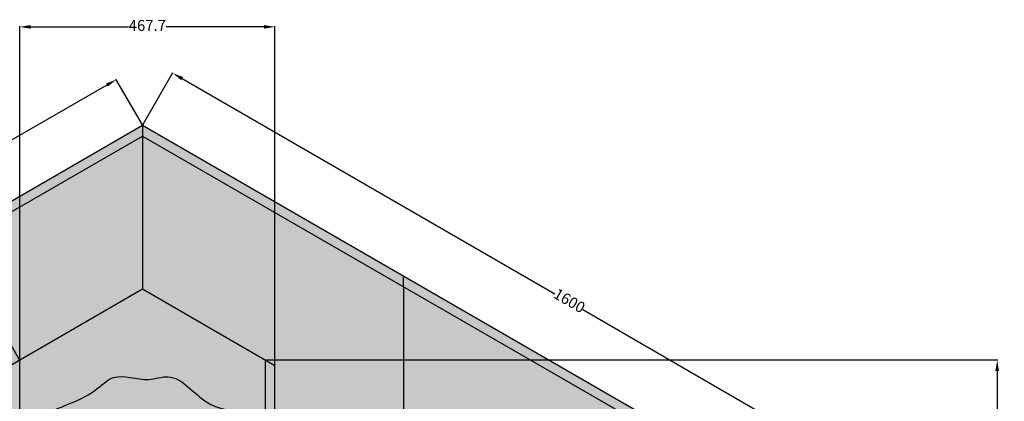
# Model space of a CAD drawing. Units: millimetres. Extents: x 78378 to 86415, y 148682 to 152721.
# Tile 16 of 18: x 80164 to 81968, y 151749 to 152448. Entities that reach past the tile are written whole.
import ezdxf

# ---------------------------------------------------------------- set-up
doc = ezdxf.new("R2010")
doc.units = ezdxf.units.MM
for name, color, linetype, lineweight in [('A-ANNO-DIMS', 2, 'Continuous', 18), ('A-FURN', 4, 'Continuous', 25), ('A-FURN-PATT', 32, 'Continuous', 13)]:
    doc.layers.add(name, color=color, linetype=linetype, lineweight=lineweight)
doc.styles.get("Standard").update_dxf_attribs({"font": 'arial.ttf'})
doc.dimstyles.new('ISO-25', dxfattribs={"dimtxt": 20, "dimasz": 20, "dimexe": 1.25, "dimexo": 0.625, "dimtad": 0, "dimdec": 1, "dimtxsty": 'Standard', "dimcen": 2.5, "dimadec": 0, "dimazin": 0, "dimtfac": 1, "dimtdec": 1, "dimtmove": 0, "dimatfit": 3, "dimfxl": 1, "dimarcsym": 0})

# ---------------------------------------------------------------- blocks, each defined once
blk = doc.blocks.new('*D2')
at = {"layer": 'A-ANNO-DIMS', "color": 0, "lineweight": -2, "transparency": 16777216}
for p, q in [((80324, 152328.4), (79430.3, 151812.5)), ((80389.2, 152255.5), (80340.7, 152339.5)), ((78540, 151298.4), (79377.3, 151781.8)), ((78570.5, 151205.5), (78522.1, 151289.5))]:
    blk.add_line(p, q, dxfattribs=at)
at = {"layer": 'A-ANNO-DIMS', "color": 0, "transparency": 16777216}
for points in [[(80322.4, 152331.3), (80325.7, 152325.6), (80341.3, 152338.4)], [(78538.3, 151301.3), (78541.7, 151295.6), (78522.7, 151288.4)]]:
    blk.add_solid(points, dxfattribs=at)
at = {"layer": 'Defpoints', "color": 0, "transparency": 16777216}
for p in [(80341.3, 152338.4), (80389.5, 152255), (78570.9, 151205)]:
    blk.add_point(p, dxfattribs=at)
at = {"layer": 'A-ANNO-DIMS', "color": 0, "transparency": 16777216, "insert": (79403.8, 151797.2), "char_height": 20, "attachment_point": 5, "rotation": 30}
blk.add_mtext('2100', dxfattribs=at)
blk = doc.blocks.new('*D3')
at = {"layer": 'A-ANNO-DIMS', "color": 0, "lineweight": -2, "transparency": 16777216}
for p, q in [((80389.8, 152255.5), (80445.2, 152351.4)), ((80461.9, 152340.3), (81144.7, 151946.1)), ((81812.9, 151560.3), (81195.8, 151916.6)), ((81775.5, 151455.5), (81830.8, 151551.4))]:
    blk.add_line(p, q, dxfattribs=at)
at = {"layer": 'A-ANNO-DIMS', "color": 0, "transparency": 16777216}
for points in [[(80463.5, 152343.2), (80460.2, 152337.4), (80444.5, 152350.3)], [(81814.5, 151563.2), (81811.2, 151557.4), (81830.2, 151550.3)]]:
    blk.add_solid(points, dxfattribs=at)
at = {"layer": 'Defpoints', "color": 0, "transparency": 16777216}
for p in [(80389.5, 152255), (81830.2, 151550.3), (81775.2, 151455)]:
    blk.add_point(p, dxfattribs=at)
at = {"layer": 'A-ANNO-DIMS', "color": 0, "transparency": 16777216, "insert": (81170.2, 151931.4), "char_height": 20, "attachment_point": 5, "rotation": 330}
blk.add_mtext('1600', dxfattribs=at)
blk = doc.blocks.new('*D17')
at = {"layer": 'A-ANNO-DIMS', "color": 0, "lineweight": -2, "transparency": 16777216}
for p, q in [((80164, 151825.5), (80073.7, 151982)), ((80057, 151970.9), (79823.5, 151836.1)), ((79550.4, 151678.4), (79783.9, 151813.2)), ((79622.8, 151513), (79532.5, 151669.5))]:
    blk.add_line(p, q, dxfattribs=at)
at = {"layer": 'A-ANNO-DIMS', "color": 0, "transparency": 16777216}
for points in [[(80055.4, 151973.8), (80058.7, 151968), (80074.3, 151980.9)], [(79548.7, 151681.3), (79552.1, 151675.5), (79533.1, 151668.4)]]:
    blk.add_solid(points, dxfattribs=at)
at = {"layer": 'Defpoints', "color": 0, "transparency": 16777216}
for p in [(80074.3, 151980.9), (80164.3, 151825), (79623.1, 151512.5)]:
    blk.add_point(p, dxfattribs=at)
at = {"layer": 'A-ANNO-DIMS', "color": 0, "transparency": 16777216, "insert": (79803.7, 151824.6), "char_height": 20, "attachment_point": 5, "rotation": 30}
blk.add_mtext('625', dxfattribs=at)
blk = doc.blocks.new('*D30')
at = {"layer": 'A-ANNO-DIMS', "color": 0, "lineweight": -2, "transparency": 16777216}
for p, q in [((80615.3, 151825), (81956.4, 151825)), ((81955.2, 151805), (81955.2, 151487.6)), ((81955.2, 151125), (81955.2, 151442.4)), ((80615.3, 151105), (81956.4, 151105))]:
    blk.add_line(p, q, dxfattribs=at)
at = {"layer": 'A-ANNO-DIMS', "color": 0, "transparency": 16777216}
for points in [[(81951.8, 151805), (81958.5, 151805), (81955.2, 151825)], [(81951.8, 151125), (81958.5, 151125), (81955.2, 151105)]]:
    blk.add_solid(points, dxfattribs=at)
at = {"layer": 'Defpoints', "color": 0, "transparency": 16777216}
for p in [(80614.7, 151825), (81955.2, 151825), (80614.7, 151105)]:
    blk.add_point(p, dxfattribs=at)
at = {"layer": 'A-ANNO-DIMS', "color": 0, "transparency": 16777216, "insert": (81955.2, 151465), "char_height": 20, "attachment_point": 5, "rotation": 90}
blk.add_mtext('720', dxfattribs=at)
blk = doc.blocks.new('*D33')
at = {"layer": 'A-ANNO-DIMS', "color": 0, "lineweight": -2, "transparency": 16777216}
for p, q in [((80164.3, 151105.6), (80164.3, 152436.3)), ((80184.3, 152435), (80363.4, 152435)), ((80612, 152435), (80432.9, 152435)), ((80632, 151105.6), (80632, 152436.3))]:
    blk.add_line(p, q, dxfattribs=at)
at = {"layer": 'A-ANNO-DIMS', "color": 0, "transparency": 16777216}
for points in [[(80184.3, 152438.3), (80184.3, 152431.7), (80164.3, 152435)], [(80612, 152438.3), (80612, 152431.7), (80632, 152435)]]:
    blk.add_solid(points, dxfattribs=at)
at = {"layer": 'Defpoints', "color": 0, "transparency": 16777216}
for p in [(80632, 152435), (80164.3, 151105), (80632, 151105)]:
    blk.add_point(p, dxfattribs=at)
at = {"layer": 'A-ANNO-DIMS', "color": 0, "transparency": 16777216, "insert": (80398.2, 152435), "char_height": 20, "attachment_point": 5}
blk.add_mtext('467.7', dxfattribs=at)

msp = doc.modelspace()

# ---------------------------------------------------------------- hatches: boundary and pattern name
at = {"layer": 'A-FURN-PATT'}
h = msp.add_hatch(color=256, dxfattribs=at)
h.dxf.hatch_style = 1
h.paths.add_polyline_path([(80389.5131, 152235.0076), (80389.5131, 152255.0076), (79662.0518, 151835.0076), (79662.0518, 151815.0076)])
h.paths.add_polyline_path([(79662.0518, 151815.0076), (79662.0518, 151835.0076), (79099.1352, 151510.0076), (79099.1352, 151490.0076)])
h.paths.add_polyline_path([(79099.1352, 151490.0076), (79099.1352, 151510.0076), (78579.52, 151210.0076), (78596.8405, 151200.0076)])
h.paths.add_polyline_path([(80632.0002, 152115.0076), (80632.0002, 152095.0076), (80867.7794, 151958.8805), (80867.7794, 151978.8805)])
h.paths.add_polyline_path([(80389.5131, 152255.0076), (80389.5131, 152235.0076), (80632.0002, 152095.0076), (80632.0002, 152115.0076)])
h = msp.add_hatch(color=256, dxfattribs=at)
h.dxf.hatch_style = 1
h.paths.add_polyline_path([(78839.3276, 151040.0076), (78579.52, 151190.0076), (78579.52, 150470.0076), (78839.3276, 150320.0076)])
h.paths.add_polyline_path([(79073.1545, 150899.6469, 0.277779695), (79002.2645, 150996.3205, 0.791083931), (78917.9567, 150978.8719, 0.180448316), (78856.6481, 150853.0138), (78856.6481, 150350.6973), (79073.1545, 150484.318)])
h.paths.add_polyline_path([(79073.1545, 151175.0076), (78856.6481, 151050.0076), (78856.6481, 150853.0138, -0.180448316), (78917.9567, 150978.8719, -0.791083931), (79002.2645, 150996.3205, -0.277779695), (79073.1545, 150899.6469)])
h.paths.add_polyline_path([(79341.6224, 151350.0076), (79099.1352, 151490.0076), (78596.8405, 151200.0076), (78839.3276, 151060.0076)])
h.paths.add_polyline_path([(79904.5389, 151675.0076), (79662.0518, 151815.0076), (79099.1352, 151490.0076), (79341.6224, 151350.0076)])
h.paths.add_polyline_path([(80389.5131, 151955.0076), (80389.5131, 152235.0076), (79662.0518, 151815.0076), (79904.5389, 151675.0076)])
h.paths.add_polyline_path([(80389.5131, 151955.0076), (80164.3465, 151825.0076), (80164.3465, 151105.0076), (80614.6797, 151105.0076), (80614.6797, 151825.0076)])
edge = h.paths.add_edge_path(flags=16)
edge.add_spline(control_points=[(80216.308, 151728.251), (80227.1854, 151732.981), (80256.3301, 151745.6544), (80298.41, 151761.9595), (80340.2597, 151805.855), (80391.0771, 151782.0404), (80454.0396, 151805.7581), (80496.5007, 151742.4095), (80543.8218, 151733.4043), (80562.7182, 151729.8083)], knot_values=[0, 0, 0, 0, 35.543746761, 95.235753469, 136.367675126, 200.932981967, 236.726410811, 322.889934976, 380.170273667, 380.170273667, 380.170273667, 380.170273667], degree=3, periodic=0)
edge.add_line((80562.7182, 151729.8083), (80562.7182, 151165.0076))
edge.add_line((80562.7182, 151165.0076), (80216.308, 151165.0076))
edge.add_line((80216.308, 151165.0076), (80216.308, 151728.251))
h.paths.add_polyline_path([(80632.0002, 152095.0076), (80389.5131, 152235.0076), (80389.5131, 151955.0076), (80614.6797, 151825.0076), (80632.0002, 151815.0076)])
h.paths.add_polyline_path([(80867.7794, 151958.8805), (80632.0002, 152095.0076), (80632.0002, 151815.0076), (80632.0002, 151510.0076), (80867.7794, 151373.8805)])
h.paths.add_polyline_path([(80147.026, 151495.8203, 0.18918979), (80063.5671, 151597.7244, 0.788261355), (79979.2691, 151580.5832, 0.160726132), (79904.5389, 151413.5769), (79904.5389, 150955.0076), (80147.026, 151095.0076)])
h.paths.add_polyline_path([(80147.026, 151815.0076), (79904.5389, 151675.0076), (79904.5389, 151413.5769, -0.160726132), (79979.2691, 151580.5832, -0.788261355), (80063.5671, 151597.7244, -0.18918979), (80147.026, 151495.8203)])
h.paths.add_polyline_path([(79887.2184, 151645.0076), (79640.4011, 151502.5076), (79640.4011, 151262.3325, -0.160726132), (79715.1313, 151429.3387, -0.788261355), (79799.4294, 151446.48, -0.21290578), (79887.2184, 151328.7247)])
h.paths.add_polyline_path([(79799.4294, 151446.48, 0.788261355), (79715.1313, 151429.3387, 0.160726132), (79640.4011, 151262.3325), (79640.4011, 150822.5076), (79887.2184, 150965.0076), (79887.2184, 151328.7247, 0.21290578)])
h.paths.add_polyline_path([(79605.7601, 151482.5076), (79358.9429, 151340.0076), (79358.9429, 151100.0701, -0.160726132), (79433.6731, 151267.0764, -0.788261355), (79517.9711, 151284.2176, -0.21290578), (79605.7601, 151166.4623)])
h.paths.add_polyline_path([(79605.7601, 151166.4623, 0.21290578), (79517.9711, 151284.2176, 0.788261355), (79433.6731, 151267.0764, 0.160726132), (79358.9429, 151100.0701), (79358.9429, 150742.9831), (79419.0877, 150694.7323), (79605.7601, 150802.5076)])
edge = h.paths.add_edge_path(flags=0)
edge.add_spline(control_points=[(81152.4356, 151098.7676), (81105.7208, 151145.9466), (81038.6136, 151213.7208), (80882.3866, 151214.1938), (80797.4434, 151311.2997), (80711.8686, 151340.3754), (80681.7691, 151350.6023)], knot_values=[0, 0, 0, 0, 188.233441, 270.4032752, 445.451792012, 540.428588287, 540.428588287, 540.428588287, 540.428588287], degree=3, periodic=0)
edge.add_line((80683.4538, 151350.0269), (80683.4538, 151104.8792))
edge.add_line((80683.4538, 151104.8792), (81152.4356, 150851.399))
edge.add_line((81152.4356, 150851.399), (81152.4356, 151098.7676))
edge = h.paths.add_edge_path(flags=0)
edge.add_spline(control_points=[(80912.9018, 151027.1103), (80892.3742, 151034.1027), (80860.1663, 151045.0739), (80835.5097, 151068.1214), (80826.5679, 151076.4797)], knot_values=[0, 0, 0, 0, 63.98405104, 100.391424282, 100.391424282, 100.391424282, 100.391424282], degree=3, periodic=0)
edge.add_arc((80830.0414, 151081.2992), 5.9407, 100.9277276, 234.2187381, ccw=False)
edge.add_spline(control_points=[(80828.9152, 151087.1322), (80837.857, 151078.7739), (80862.5136, 151055.7263), (80894.7215, 151044.7552), (80915.2491, 151037.7628)], knot_values=[0, 0, 0, 0, 36.407373242, 100.391424282, 100.391424282, 100.391424282, 100.391424282], degree=3, periodic=0)
edge.add_arc((80914.7882, 151032.2795), 5.5026, -107.9540399, 85.195579, ccw=False)
h.paths.add_polyline_path([(81238.218, 151110.0076), (80632.0002, 151460.0076), (80632.0002, 151105.0076), (81238.218, 150755.0076)])
edge = h.paths.add_edge_path(flags=16)
edge.add_line((81152.4356, 150851.399), (80683.4538, 151104.8792))
edge.add_line((80683.4538, 151104.8792), (80683.4538, 151350.0279))
edge.add_spline(control_points=[(80681.7691, 151350.6023), (80711.8686, 151340.3754), (80797.4434, 151311.2997), (80882.3866, 151214.1938), (81038.6136, 151213.7208), (81105.7208, 151145.9466), (81152.4356, 151098.7676)], knot_values=[0, 0, 0, 0, 94.976796275, 270.025313088, 352.195147288, 540.428588287, 540.428588287, 540.428588287, 540.428588287], degree=3, periodic=0)
edge.add_line((81152.4356, 151098.7676), (81152.4356, 150851.399))
edge = h.paths.add_edge_path(flags=0)
edge.add_spline(control_points=[(80912.9018, 151027.1103), (80892.3742, 151034.1027), (80860.1663, 151045.0739), (80835.5097, 151068.1214), (80826.5679, 151076.4797)], knot_values=[0, 0, 0, 0, 63.98405104, 100.391424282, 100.391424282, 100.391424282, 100.391424282], degree=3, periodic=0)
edge.add_arc((80830.0414, 151081.2992), 5.9407, 100.9277276, 234.2187381, ccw=False)
edge.add_spline(control_points=[(80828.9152, 151087.1322), (80837.857, 151078.7739), (80862.5136, 151055.7263), (80894.7215, 151044.7552), (80915.2491, 151037.7628)], knot_values=[0, 0, 0, 0, 36.407373242, 100.391424282, 100.391424282, 100.391424282, 100.391424282], degree=3, periodic=0)
edge.add_arc((80914.7882, 151032.2795), 5.5026, -107.7417882, 85.195579, ccw=False)
h.paths.add_polyline_path([(81498.0256, 151255.0076), (81238.218, 151110.0076), (81238.218, 150755.0076), (81498.0256, 150905.0076)])
edge = h.paths.add_edge_path(flags=16)
edge.add_spline(control_points=[(81152.4356, 151098.7676), (81105.7208, 151145.9466), (81038.6136, 151213.7208), (80882.3866, 151214.1938), (80797.4434, 151311.2997), (80711.8686, 151340.3754), (80681.7691, 151350.6023)], knot_values=[0, 0, 0, 0, 188.233441, 270.4032752, 445.451792012, 540.428588287, 540.428588287, 540.428588287, 540.428588287], degree=3, periodic=0)
edge.add_line((80683.4538, 151350.0279), (80683.4538, 151104.8792))
edge.add_line((80683.4538, 151104.8792), (81152.4356, 150851.399))
edge.add_line((81152.4356, 150851.399), (81152.4356, 151098.7676))
h.paths.add_polyline_path([(81453.9904, 151280.4314), (80867.7794, 151618.8805), (80867.7794, 151373.8805), (81238.218, 151160.0076)])
edge = h.paths.add_edge_path(flags=16)
edge.add_line((81189.2304, 151297.6373), (81114.4166, 151300.2154))
edge.add_arc((81412.0967, 151394.0167), 312.1092, 179.7569303, 197.4900342, ccw=False)
edge.add_ellipse((81154.0183, 151392.0436), major_axis=(-54.0264, 3.6301), ratio=0.221796934, start_angle=0, end_angle=0.3517985, ccw=False)
edge.add_ellipse((81154.0183, 151392.0436), major_axis=(-54.0264, 3.6301), ratio=0.221796934, start_angle=180, end_angle=360, ccw=False)
edge.add_spline(control_points=[(81196.1844, 151321.9476), (81224.9802, 151347.1455), (81266.8846, 151383.8144), (81222.0354, 151387.0304), (81208.0056, 151388.0364)], knot_values=[0, 0, 0, 0, 75.091751734, 109.275804387, 109.275804387, 109.275804387, 109.275804387], degree=3, periodic=0)
edge.add_arc((80751.9112, 151435.6145), 458.5693, 342.4891602, 345.646172, ccw=False)
edge = h.paths.add_edge_path(flags=0)
edge.add_spline(control_points=[(81196.6193, 151323.657), (81197.893, 151324.7717), (81199.1654, 151325.8858), (81209.0233, 151334.5343), (81217.3959, 151341.9835), (81228.0928, 151352.5012), (81231.3883, 151355.9524), (81236.9493, 151362.4395), (81239.214, 151365.4773), (81241.4987, 151369.416), (81242.064, 151370.5542), (81242.9187, 151372.6971), (81243.2076, 151373.7015), (81243.5012, 151375.5539), (81243.5065, 151376.4), (81243.2432, 151377.9407), (81242.9775, 151378.6373), (81242.1402, 151379.937), (81241.5659, 151380.5416), (81240.2039, 151381.533), (81239.4963, 151381.9384), (81237.0619, 151383.0663), (81235.0242, 151383.6999), (81230.352, 151384.7569), (81227.7173, 151385.1826), (81221.9118, 151385.9145), (81218.7193, 151386.2133), (81213.7912, 151386.6115), (81212.1252, 151386.7359), (81209.6196, 151386.9181), (81208.7865, 151386.9779), (81207.9009, 151387.0432)], knot_values=[0.015487437, 0.015487437, 0.015487437, 0.015487437, 3.337879569, 3.337879569, 25.851306242, 25.851306242, 37.52811308, 37.52811308, 49.204919918, 49.204919918, 54.285093801, 54.285093801, 59.365267683, 59.365267683, 64.445441566, 64.445441566, 69.525615449, 69.525615449, 74.605789331, 74.605789331, 78.493667847, 78.493667847, 86.255670953, 86.255670953, 94.017674059, 94.017674059, 102.202265559, 102.202265559, 106.294561309, 106.294561309, 108.325221747, 108.325221747, 108.325221747, 108.325221747], degree=3, periodic=0)
edge = h.paths.add_edge_path(flags=16)
edge.add_arc((81034.1732, 151350.4693), 42.5822, 231.2679035, 306.151846, ccw=False)
edge.add_line((81007.5303, 151317.2517), (81007.5303, 151395.181))
edge.add_ellipse((81033.412, 151394.7791), major_axis=(-25.8816, 0.4538), ratio=0.23894509, start_angle=0, end_angle=0.1147075, ccw=False)
edge.add_ellipse((81033.412, 151394.7791), major_axis=(-25.8816, 0.4538), ratio=0.23894509, start_angle=181.1677709, end_angle=358.9476457, ccw=False)
edge.add_ellipse((81033.412, 151395.7791), major_axis=(-25.8816, 0.4538), ratio=0.23894509, start_angle=180, end_angle=360.1147075, ccw=False)
edge.add_ellipse((81033.412, 151395.7791), major_axis=(-25.8816, 0.4538), ratio=0.23894509, start_angle=178.9476457, end_angle=180, ccw=False)
edge.add_line((81059.2936, 151395.1778), (81059.2936, 151394.3772))
edge.add_ellipse((81033.412, 151394.7791), major_axis=(-25.8816, 0.4538), ratio=0.23894509, start_angle=180, end_angle=180.1147075, ccw=False)
edge.add_ellipse((81033.412, 151394.7791), major_axis=(-25.8816, 0.4538), ratio=0.23894509, start_angle=3.6903098, end_angle=176.4406503, ccw=False)
edge.add_line((81059.2936, 151393.3388), (81059.2936, 151316.086))
h.paths.add_polyline_path([(80951.9355, 151343.9568), (80909.6838, 151362.4635), (80904.0219, 151443.9615, -0.381333076), (80987.2169, 151411.3717)], flags=16)
h = msp.add_hatch(color=256, dxfattribs=at)
h.dxf.hatch_style = 1
h.paths.add_polyline_path([(80867.7794, 151978.8805), (80867.7794, 151958.8805), (81766.4935, 151440.0076), (81766.4935, 150140.0076), (81775.1537, 150135.0076), (81775.1537, 151455.0076)])
h = msp.add_hatch(color=256, dxfattribs=at)
h.dxf.hatch_style = 1
h.paths.add_polyline_path([(80389.8136, 150935.1811), (80389.5131, 151105.0076), (80164.3465, 151105.0076), (79904.5389, 150955.0076), (79433.5848, 150683.1022), (79459.4128, 150662.3818), (79243.9048, 150537.9582), (79160.4069, 150518.1674), (78839.3276, 150320.0076), (78579.52, 150470.0076), (78570.8597, 150475.0076), (78570.8597, 150465.0076), (78570.8597, 149885.0076)])
h.paths.add_polyline_path([(80086.4042, 150460.0076), (79826.5966, 150610.0076), (78570.8597, 149885.0076), (78830.6674, 149735.0076)])
h.paths.add_polyline_path([(79540.8001, 150161.0557), (79217.3967, 149974.3386), (78980.9166, 150110.8705), (79304.32, 150297.5875)], flags=16)
h.paths.add_polyline_path([(79506.159, 150161.0557), (79217.3967, 149994.3386), (79015.5576, 150110.8705), (79304.32, 150277.5875)], flags=0)
edge = h.paths.add_edge_path(flags=0)
edge.add_arc((79247.8636, 150177.1541), 137.9799, 256.0025928, 293.5594109)
edge.add_arc((79240.7671, 150078.2605), 68.0855, 336.099104, 387.3696877)
edge.add_ellipse((79258.3074, 150109.4852), major_axis=(-42.6234, -1.6591), ratio=0.160428429, start_angle=0, end_angle=179.0977279, ccw=False)
edge.add_arc((79285.2112, 150074.2509), 77.2096, 155.1233104, 203.6557939)
edge = h.paths.add_edge_path(flags=0)
edge.add_ellipse((79258.6958, 150110.8297), major_axis=(-42.6234, -1.6591), ratio=0.160428429, start_angle=350.6039412, end_angle=356.2289762)
edge.add_line((79219.169, 150111.8937), (79218.3268, 150109.4141))
edge.add_arc((79262.4675, 150032.9602), 88.2813, 112.3931229, 120, ccw=False)
h.paths.add_polyline_path([(79287.0625, 150086.9703, -0.247702064), (79288.1967, 150077.2955, -0.390476513), (79265.4731, 150072.5438, -0.487261526), (79264.079, 150082.3769, 0.395604326)], flags=0)
h.paths.add_polyline_path([(80389.5131, 150935.0076), (79826.5966, 150610.0076), (80086.4042, 150460.0076), (80692.622, 150460.0076), (80952.4296, 150610.0076)])
edge = h.paths.add_edge_path(flags=16)
edge.add_ellipse((80392.4466, 150825.601), major_axis=(-133.0757, 7.722), ratio=0.42449957, start_angle=0, end_angle=360)
edge = h.paths.add_edge_path(flags=0)
edge.add_spline(control_points=[(80269.3541, 150832.7436), (80269.2919, 150831.672), (80269.3503, 150830.5922), (80269.7341, 150828.3361), (80270.0612, 150827.1587), (80271.0461, 150824.6748), (80271.7052, 150823.3692), (80273.4061, 150820.6503), (80274.4481, 150819.2381), (80276.9366, 150816.3509), (80278.3828, 150814.8762), (80282.5858, 150811.0913), (80285.6261, 150808.7701), (80292.6031, 150804.2267), (80296.5388, 150802.0041), (80305.195, 150797.7581), (80309.9151, 150795.7344), (80320.0112, 150791.96), (80325.387, 150790.2092), (80339.2162, 150786.315), (80347.9578, 150784.3563), (80366.0679, 150781.2568), (80375.4359, 150780.1158), (80394.3093, 150778.7158), (80403.8142, 150778.4568), (80422.4656, 150778.8319), (80431.6115, 150779.4662), (80449.0608, 150781.5838), (80457.3636, 150783.0675), (80472.6699, 150786.7766), (80479.6726, 150789.0033), (80490.1894, 150793.2813), (80494.1268, 150795.1967), (80501.0146, 150799.1885), (80503.9632, 150801.2651), (80508.2066, 150804.9015), (80509.73, 150806.4609), (80512.1996, 150809.4942), (80513.1456, 150810.9657), (80514.4291, 150813.5431), (80514.8436, 150814.6688), (80515.3984, 150816.8625), (80515.5405, 150817.9315), (80515.5801, 150820.098), (80515.4773, 150821.1978), (80514.9905, 150823.5062), (80514.6047, 150824.7154), (80513.4854, 150827.2641), (80512.7511, 150828.6027), (80510.8872, 150831.3809), (80509.7578, 150832.8196), (80507.0873, 150835.7513), (80505.5466, 150837.2439), (80501.0624, 150841.0944), (80497.8199, 150843.4576), (80490.4174, 150848.062), (80486.2582, 150850.3037), (80477.1448, 150854.5643), (80472.1909, 150856.5835), (80461.6275, 150860.3245), (80456.0182, 150862.0465), (80441.7332, 150865.8127), (80432.7885, 150867.6675), (80414.3391, 150870.5317), (80404.8349, 150871.5411), (80385.7707, 150872.6572), (80376.2113, 150872.764), (80357.5444, 150872.0728), (80348.4375, 150871.2748), (80331.1682, 150868.83), (80323.0064, 150867.1827), (80309.472, 150863.5363), (80303.8628, 150861.6593), (80293.8018, 150857.5401), (80289.3512, 150855.2969), (80282.7757, 150851.2345), (80280.3473, 150849.4579), (80276.2606, 150845.9127), (80274.604, 150844.1458), (80272.3157, 150841.1243), (80271.5358, 150839.8454), (80270.3496, 150837.3879), (80269.9417, 150836.2101), (80269.5065, 150834.2815), (80269.3988, 150833.5143), (80269.3541, 150832.7436)], knot_values=[0, 0, 0, 0, 0.09750046, 0.09750046, 0.19500092, 0.19500092, 0.292501379, 0.292501379, 0.390001839, 0.390001839, 0.487502299, 0.487502299, 0.638803224, 0.638803224, 0.790104149, 0.790104149, 0.941405074, 0.941405074, 1.092705999, 1.092705999, 1.312817101, 1.312817101, 1.532928203, 1.532928203, 1.753039304, 1.753039304, 1.973150406, 1.973150406, 2.193261508, 2.193261508, 2.413372609, 2.413372609, 2.569860633, 2.569860633, 2.726348657, 2.726348657, 2.844186582, 2.844186582, 2.962024507, 2.962024507, 3.060233876, 3.060233876, 3.158443245, 3.158443245, 3.256652615, 3.256652615, 3.354861984, 3.354861984, 3.453071354, 3.453071354, 3.551280723, 3.551280723, 3.649490093, 3.649490093, 3.80392773, 3.80392773, 3.958365368, 3.958365368, 4.112803006, 4.112803006, 4.267240644, 4.267240644, 4.489203495, 4.489203495, 4.711166346, 4.711166346, 4.933129197, 4.933129197, 5.155092048, 5.155092048, 5.3770549, 5.3770549, 5.557853609, 5.557853609, 5.738652318, 5.738652318, 5.872395556, 5.872395556, 6.006138794, 6.006138794, 6.109604996, 6.109604996, 6.213071198, 6.213071198, 6.283185307, 6.283185307, 6.283185307, 6.283185307], degree=3, periodic=0)
edge = h.paths.add_edge_path(flags=0)
edge.add_ellipse((80392.4466, 150825.601), major_axis=(-101.8398, 3.3923), ratio=0.403492477, start_angle=0, end_angle=360)
edge = h.paths.add_edge_path(flags=0)
edge.add_ellipse((80391.1657, 150858.3746), major_axis=(9.0882, -0.6733), ratio=0.351354129, start_angle=0, end_angle=360)
h.paths.add_polyline_path([(80952.4296, 150610.0076), (80692.622, 150460.0076), (81361.2342, 150073.9842), (81649.9628, 150052.7286), (81766.4935, 150120.0076), (81766.4935, 150140.0076), (81564.9025, 150256.3963), (81564.8884, 150096.1963), (81538.9076, 150111.1963), (81538.9217, 150271.3963)])
h.paths.add_polyline_path([(81539.0357, 151571.3305), (80867.7794, 151958.8805), (80867.7794, 151618.8805), (81498.0256, 151255.0076), (81498.0256, 150905.0076), (81238.218, 150755.0076), (81538.9488, 150581.3806)])
h.paths.add_polyline_path([(81766.4935, 151440.0076), (81565.0164, 151556.3305), (81564.9296, 150566.3806), (81766.4935, 150450.0076)])
edge = h.paths.add_edge_path()
edge.add_line((81564.9296, 150566.3806), (81564.9137, 150384.6289))
edge.add_ellipse((81552.1304, 150358.5718), major_axis=(52.6272, 3.506), ratio=0.495899055, start_angle=367.5169757, end_angle=420.0564686, ccw=False)
edge.add_ellipse((81552.1304, 150358.5718), major_axis=(52.6272, 3.506), ratio=0.495899055, start_angle=351.729742, end_angle=367.5169757, ccw=False)
edge.add_ellipse((81552.1304, 150345.5016), major_axis=(52.6272, 3.506), ratio=0.495899055, start_angle=352.5116949, end_angle=366.3006092, ccw=False)
edge.add_line((81603.4463, 150342.2039), (81603.5064, 150340.4475))
edge.add_ellipse((81552.1304, 150332.128), major_axis=(52.6272, 3.506), ratio=0.495899055, start_angle=353.6729654, end_angle=365.3867997, ccw=False)
edge.add_ellipse((81552.1304, 150332.128), major_axis=(52.6272, 3.506), ratio=0.495899055, start_angle=350.9388331, end_angle=353.6729654)
edge.add_line((81603.8688, 150329.855), (81604.0442, 150324.7302))
edge.add_ellipse((81552.1304, 150317.7418), major_axis=(52.6272, 3.506), ratio=0.495899055, start_angle=355.2176746, end_angle=363.8553364, ccw=False)
edge.add_ellipse((81552.1304, 150317.7418), major_axis=(52.6272, 3.506), ratio=0.495899055, start_angle=341.3250873, end_angle=355.2176746, ccw=False)
edge.add_ellipse((81552.1304, 150317.7418), major_axis=(52.6272, 3.506), ratio=0.495899055, start_angle=293.4661701, end_angle=341.3250873, ccw=False)
edge.add_line((81564.9057, 150292.9664), (81564.9025, 150256.3963))
edge.add_line((81564.9025, 150256.3963), (81766.4935, 150140.0076))
edge.add_line((81766.4935, 150140.0076), (81766.4935, 150450.0076))
edge.add_line((81766.4935, 150450.0076), (81564.9296, 150566.3806))
h.paths.add_polyline_path([(81525.5713, 150321.598), (81526.5985, 150321.3069), (81528.6771, 150320.947)])
h.paths.add_polyline_path([(81512.7903, 150326.1129), (81514.5058, 150325.3887), (81512.538, 150326.2678)])
h.paths.add_polyline_path([(81533.2148, 150320.1615), (81534.6952, 150319.9052), (81536.5995, 150319.7557)])
h.paths.add_polyline_path([(81518.622, 150323.6513), (81519.227, 150323.3959), (81521.289, 150322.8116)])
h.paths.add_polyline_path([(81501.2183, 150336.2599), (81500.3543, 150338.1339), (81499.7815, 150340.0494), (81499.5032, 150341.9955), (81499.5032, 150343.7257), (81499.7584, 150345.5905), (81500.2766, 150347.4549), (81501.0551, 150349.3095), (81501.0967, 150349.3937), (81501.1389, 150349.4778), (81500.9978, 150349.7496), (81500.8628, 150350.0225), (81499.5032, 150355.0658), (81499.9591, 150359.5002), (81501.8982, 150363.9083), (81505.2653, 150368.1646), (81509.9647, 150372.1482), (81515.8627, 150375.7459), (81522.7918, 150378.8553), (81530.555, 150381.3882), (81538.9315, 150383.2724), (81538.9488, 150581.3806), (80632.0002, 151105.0076), (80389.5131, 151105.0076), (80389.8142, 150934.8338), (80952.4296, 150610.0076), (81538.9217, 150271.3963), (81538.9234, 150291.7194), (81538.8752, 150291.721), (81530.1915, 150292.8239), (81522.1802, 150294.6904), (81515.0866, 150297.2633), (81509.8635, 150299.9959), (81505.6084, 150303.1351), (81502.419, 150306.6088), (81500.3683, 150310.3375), (81499.5032, 150314.2358), (81499.5032, 150315.9659), (81499.8206, 150318.1159), (81500.487, 150320.2634), (81501.4979, 150322.3941), (81500.487, 150324.4233), (81499.8206, 150326.5039), (81499.5032, 150328.622), (81499.5032, 150330.3521), (81499.7815, 150332.3262), (81500.3543, 150334.2992)])
h = msp.add_hatch(color=256, dxfattribs=at)
h.dxf.hatch_style = 1
h.paths.add_polyline_path([(79090.475, 151205.0076), (78839.3276, 151060.0076), (78839.3276, 150320.0076), (79090.475, 150475.0076)])
h.paths.add_polyline_path([(79073.1545, 151175.0076), (79073.1545, 150899.6469, -0.04544363), (79073.1545, 150878.5653), (79073.1545, 150484.318), (78856.6481, 150350.6973), (78856.6481, 150814.5249, -0.048157161), (78856.6481, 150853.0138), (78856.6481, 151050.0076)], flags=16)
h.paths.add_polyline_path([(79358.9429, 151340.0076), (79605.7601, 151482.5076), (79605.7601, 150802.5076), (79419.0877, 150694.7323), (79433.5848, 150683.1022), (79623.0806, 150792.5076), (79623.0806, 151512.5076), (79341.6224, 151350.0076), (79341.6224, 150756.8784), (79358.9429, 150742.9831)])
h.paths.add_polyline_path([(79341.6224, 151350.0076), (79090.475, 151205.0076), (79090.475, 150475.0076), (79160.4069, 150518.1674), (79107.7955, 150505.6973), (79107.7955, 151195.0076), (79109.5275, 151196.0076), (79324.3018, 151320.0076), (79324.3018, 150770.7736), (79341.6224, 150756.8784)])
h.paths.add_polyline_path([(79887.2184, 151645.0076), (79887.2184, 151665.0076), (79623.0806, 151512.5076), (79623.0806, 150792.5076), (79887.2184, 150945.0076), (79887.2184, 150965.0076), (79640.4011, 150822.5076), (79640.4011, 151502.5076)])
h.paths.add_polyline_path([(79904.5389, 151655.0076), (79887.2184, 151645.0076), (79887.2184, 150965.0076), (79904.5389, 150975.0076)])
h.paths.add_polyline_path([(80164.3465, 151825.0076), (80147.026, 151815.0076), (80147.026, 151095.0076), (80164.3465, 151105.0076)])
h.paths.add_polyline_path([(80632.0002, 151510.0076), (80632.0002, 151490.0076), (81238.218, 151140.0076), (81471.6045, 151270.2619), (81453.9904, 151280.4314), (81238.218, 151160.0076)])
h.paths.add_polyline_path([(80632.0002, 151490.0076), (80632.0002, 151470.0076), (81238.218, 151120.0076), (81489.2186, 151260.0924), (81471.6045, 151270.2619), (81238.218, 151140.0076)])
h.paths.add_polyline_path([(80632.0002, 151460.0076), (80632.0002, 151105.0076), (81238.218, 150755.0076), (81238.218, 151110.0076)])
edge = h.paths.add_edge_path(flags=16)
edge.add_spline(control_points=[(80681.7691, 151350.6023), (80711.8686, 151340.3754), (80797.4434, 151311.2997), (80882.3866, 151214.1938), (81038.6136, 151213.7208), (81105.7208, 151145.9466), (81152.4356, 151098.7676)], knot_values=[0, 0, 0, 0, 94.976796275, 270.025313088, 352.195147288, 540.428588287, 540.428588287, 540.428588287, 540.428588287], degree=3, periodic=0)
edge.add_line((81152.4356, 151098.7676), (81152.4356, 150851.399))
edge.add_line((81152.4356, 150851.399), (80683.4538, 151104.8792))
edge.add_line((80683.4538, 151104.8792), (80683.4538, 151350.027))
edge = h.paths.add_edge_path(flags=0)
edge.add_spline(control_points=[(80828.9152, 151087.1322), (80837.857, 151078.7739), (80862.5136, 151055.7263), (80894.7215, 151044.7552), (80915.2491, 151037.7628)], knot_values=[0, 0, 0, 0, 36.407373242, 100.391424282, 100.391424282, 100.391424282, 100.391424282], degree=3, periodic=0)
edge.add_arc((80914.7882, 151032.2795), 5.5026, -107.9540399, 85.195579, ccw=False)
edge.add_spline(control_points=[(80912.9018, 151027.1103), (80892.3742, 151034.1027), (80860.1663, 151045.0739), (80835.5097, 151068.1214), (80826.5679, 151076.4797)], knot_values=[0, 0, 0, 0, 63.98405104, 100.391424282, 100.391424282, 100.391424282, 100.391424282], degree=3, periodic=0)
edge.add_arc((80830.0414, 151081.2992), 5.9407, 100.9277276, 234.2187381, ccw=False)
h.paths.add_polyline_path([(80632.0002, 151815.0076), (80614.6797, 151825.0076), (80614.6797, 151105.0076), (80632.0002, 151105.0076)])
h.paths.add_polyline_path([(81498.0256, 151255.0076), (81489.2186, 151260.0924), (81238.218, 151120.0076), (80632.0002, 151470.0076), (80632.0002, 151460.0076), (81238.218, 151110.0076)])
h.paths.add_polyline_path([(78596.8405, 151200.0076), (78579.52, 151190.0076), (78839.3276, 151040.0076), (78839.3276, 151060.0076)])
h.paths.add_polyline_path([(78596.8405, 151200.0076), (78579.52, 151210.0076), (78579.52, 151190.0076)])
h.paths.add_polyline_path([(78579.52, 151210.0076), (78570.8597, 151205.0076), (78570.8597, 150475.0076), (78579.52, 150470.0076)])
h = msp.add_hatch(color=256, dxfattribs=at)
h.dxf.hatch_style = 1
h.set_gradient(color1=(255, 255, 255), color2=(199, 200, 202))
edge = h.paths.add_edge_path()
edge.add_spline(control_points=[(80562.7182, 151729.8083), (80543.8218, 151733.4043), (80496.5007, 151742.4095), (80454.0396, 151805.7581), (80391.0771, 151782.0404), (80340.2597, 151805.855), (80298.41, 151761.9595), (80256.3301, 151745.6544), (80227.1854, 151732.981), (80216.308, 151728.251)], knot_values=[0, 0, 0, 0, 57.280338691, 143.443862856, 179.2372917, 243.802598541, 284.934520198, 344.626526906, 380.170273667, 380.170273667, 380.170273667, 380.170273667], degree=3, periodic=0)
edge.add_line((80216.308, 151728.251), (80216.308, 151165.0076))
edge.add_line((80216.308, 151165.0076), (80562.7182, 151165.0076))
edge.add_line((80562.7182, 151165.0076), (80562.7182, 151729.8083))

# ---------------------------------------------------------------- linework, layer by layer
at = {"layer": 'A-FURN'}
for p, q in [((78570.8597, 151205.0076), (80389.5131, 152255.0076)), ((80389.5131, 152255.0076), (80389.5131, 151955.0076)), ((80389.5131, 152255.0076), (81775.1537, 151455.0076)), ((78579.52, 151190.0076), (80389.5131, 152235.0076)), ((80389.5131, 152235.0076), (81766.4935, 151440.0076)), ((80632.0002, 152095.0076), (80632.0002, 152115.0076)), ((80632.0002, 151105.0076), (80632.0002, 152095.0076)), ((80867.7794, 151958.8805), (80867.7794, 151978.8805)), ((79904.5389, 151675.0076), (80389.5131, 151955.0076)), ((80389.5131, 151955.0076), (80632.0002, 151815.0076)), ((80867.7794, 151958.8805), (80867.7794, 151373.8805)), ((80614.6797, 151105.0076), (80614.6797, 151825.0076))]:
    msp.add_line(p, q, dxfattribs=at)
msp.add_open_spline([(80216.308, 151728.251), (80227.1854, 151732.981), (80256.3301, 151745.6544), (80298.41, 151761.9595), (80340.2597, 151805.855), (80391.0771, 151782.0404), (80454.0396, 151805.7581), (80496.5007, 151742.4095), (80543.8218, 151733.4043), (80562.7182, 151729.8083)], degree=3, knots=[0, 0, 0, 0, 35.543746761, 95.235753469, 136.367675126, 200.932981967, 236.726410811, 322.889934976, 380.170273667, 380.170273667, 380.170273667, 380.170273667], dxfattribs=at)

# ---------------------------------------------------------------- dimensions: what is measured, and where the dimension line sits
at = {"layer": 'A-ANNO-DIMS'}
dim = msp.add_linear_dim(base=(80632.0002, 152435.0076), p1=(80164.3465, 151105.0076), p2=(80632.0002, 151105.0076), dimstyle='ISO-25', override={"dimdec": 1, "dimlfac": 1, "dimrnd": 0, "dimzin": 0, "dimdsep": 46, "dimlunit": 2}, dxfattribs=at)
dim.commit()
dim.dimension.update_dxf_attribs({"geometry": '*D33', "text_midpoint": (80398.1733, 152435.0076)})
for base, p1, p2, angle, picture, middle in [((81830.1884, 151550.3305), (80389.5131, 152255.0076), (81775.1537, 151455.0076), 330, '*D3', (81170.2376, 151931.3533)), ((80341.3443, 152338.4385), (78570.8597, 151205.0076), (80389.5131, 152255.0076), 30, '*D2', (79403.8116, 151797.1537))]:
    dim = msp.add_linear_dim(base=base, p1=p1, p2=p2, angle=angle, dimstyle='ISO-25', override={"dimclrd": 0, "dimclre": 0, "dimclrt": 0}, dxfattribs=at)
    dim.commit()
    dim.dimension.update_dxf_attribs({"geometry": picture, "text_midpoint": middle, "dimtype": 161})
for base, p1, p2, angle, picture, middle in [((80074.3465, 151980.8922), (79623.0806, 151512.5076), (80164.3465, 151825.0076), 30, '*D17', (79803.7135, 151824.6422)), ((81955.1537, 151825.0076), (80614.6797, 151105.0076), (80614.6797, 151825.0076), 90, '*D30', (81955.1537, 151465.0076))]:
    dim = msp.add_linear_dim(base=base, p1=p1, p2=p2, angle=angle, dimstyle='ISO-25', override={"dimdec": 0, "dimlfac": 1, "dimrnd": 0, "dimzin": 0, "dimdsep": 46, "dimlunit": 2}, dxfattribs=at)
    dim.commit()
    dim.dimension.update_dxf_attribs({"geometry": picture, "text_midpoint": middle})

doc.saveas('drawing.dxf')
